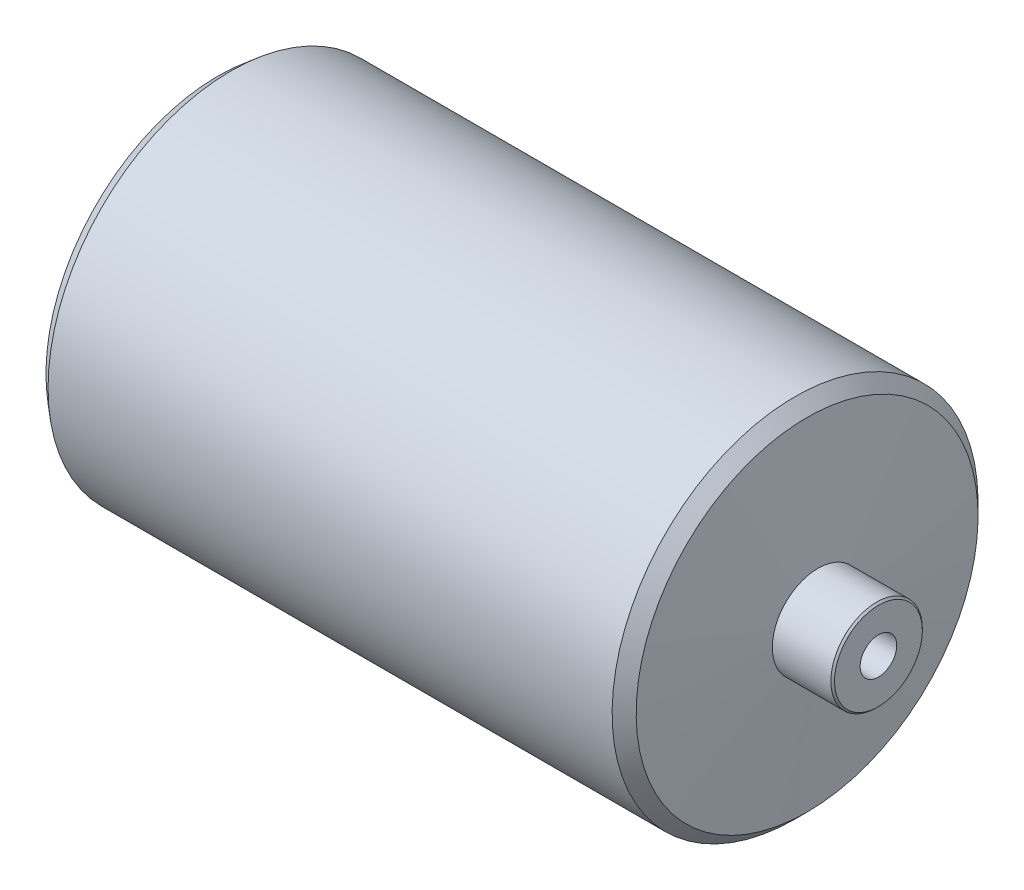
SolidWorks part; units mm, degrees
material "Plain Carbon Steel"
ref_plane "Front Plane" through (0, 0, 0) normal (0, 0, 1) x (1, 0, 0)
ref_plane "Top Plane" through (0, 0, 0) normal (0, 1, 0) x (1, 0, 0)
ref_plane "Right Plane" through (0, 0, 0) normal (1, 0, 0) x (0, 0, -1)
sketch "Roller Profile Sketch" plane through (0, 0, 0) normal (0, 0, 1) x (1, 0, 0)
  line L0 (0, 0) -> (0, 12.5)
  line L1 (0, 12.5) -> (16.5, 12.5)
  line L2 (16.5, 12.5) -> (19.7808, 50)
  line L3 (19.7808, 50) -> (180.2192, 50)
  line L4 (180.2192, 50) -> (183.5, 12.5)
  line L5 (183.5, 12.5) -> (200, 12.5)
  line L6 (200, 12.5) -> (200, 0)
  line L7 (200, 0) -> (0, 0)
  dimension "D1" = 50
  dimension "D2" = 12.5
  dimension "D3" = 200
  dimension "D4" = 16.5
  dimension "D5" = 16.5
  dimension "D6" = 85
  dimension "D7" = 85
revolve "Roller Body" add sketch "Roller Profile Sketch" angle 360 about L7
chamfer "Journal Chamfer 0.5mm A" distance 0.5 angle 45 1 edges at (200, 12.5, 0)
chamfer "Journal Chamfer 0.5mm B" distance 0.5 angle 45 1 edges at (0, 12.5, 0)
chamfer "Body Edge Chamfer 3mm" distance 3 angle 45 2 edges at (19.7808, 50, 0) (180.2192, 50, 0)
hole_wizard "Centre Hole Ø10x59 End A" positions "Sketch2" profile "Sketch3" legacy
sketch "Sketch2" plane through (200, 0, 0) normal (1, 0, 0) x (0, 0, -1)
  circle A0 centre (0, 0) radius 3.2819
  point P1 (0, 0)
sketch "Sketch3" plane through (200, 0, 0) normal (0, 1, 0) x (0, 0, -1)
  line L0 (0, 0) -> (0, 59)
  line L1 (0, 59) -> (5, 59)
  line L2 (5, 59) -> (5, 0)
  line L3 (5, 0) -> (0, 0)
  line L4 (0, 110) -> (0, -10) construction
  dimension "Diameter" = 10
  dimension "Depth" = 59
hole_wizard "Centre Hole Ø10x59 End B" positions "Sketch4" profile "Sketch5" legacy
sketch "Sketch4" plane through (0, 0, 0) normal (-1, 0, 0) x (0, 0, 1)
  point P0 (0, 0)
sketch "Sketch5" plane through (0, 0, 0) normal (0, 1, 0) x (0, 0, 1)
  line L0 (0, 0) -> (0, 59)
  line L1 (0, 59) -> (5, 59)
  line L2 (5, 59) -> (5, 0)
  line L3 (5, 0) -> (0, 0)
  line L4 (0, 110) -> (0, -10) construction
  dimension "Diameter" = 10
  dimension "Depth" = 59
